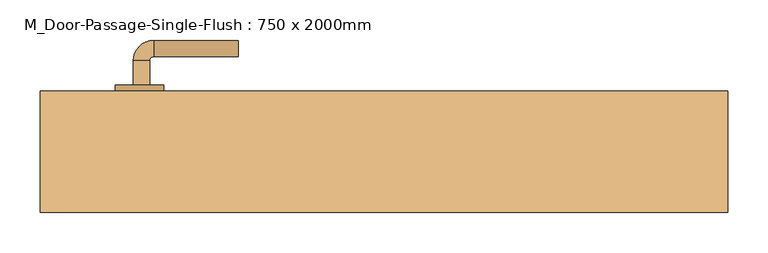
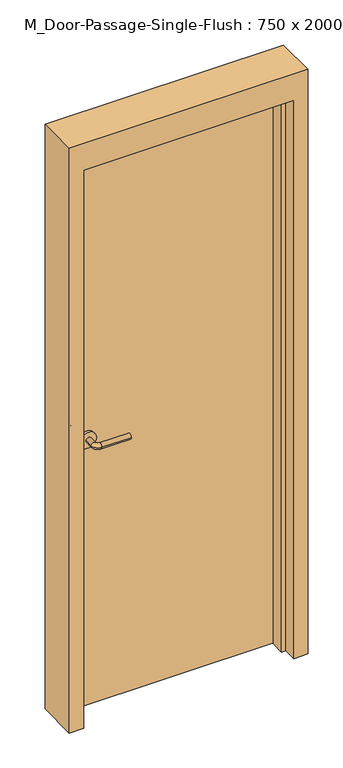
"""IFC4 building model written with IfcOpenShell, lengths in millimetres: door geometry, M_Door-Passage-Single-Flush : 750 x 2000mm."""

from ifc_helpers import new_model, si_unit, point, frame, frame_2d, origin, origin_with_axes, place, context, project, spatial, polyline, circle_curve, ellipse_curve, trimmed, segment, composite_curve, outline, extrude, faceted_brep, source, transform, mapped, element, save
from ifc_brep_helpers import plane_surface, cylinder_surface, revolved_surface, advanced_brep


def m_door_passage_single_flush_750_x_2000mm_58848773(model_context):
    return source(origin(), model_context, "Body", "SolidModel", [
        advanced_brep(
        [(-309.990625, 40.85, 1000.0), (-289.990625, 40.85, 1000.0), (-289.990625, 10.85, 1000.0), (-309.990625, 10.85, 1000.0), (-284.990625, 5.85, 1000.0), (-284.990625, -14.15, 1000.0), (-179.990625, -14.15, 1000.0), (-179.990625, 5.85, 1000.0)],
        [
            (0, 1, circle_curve(frame((-299.990625, 40.85, 1000.0), z_axis=(0.0, 1.0, 0.0), x_axis=(1.0, 0.0, 0.0)), 10.0)),
            (1, 0, circle_curve(frame((-299.990625, 40.85, 1000.0), z_axis=(0.0, 1.0, 0.0), x_axis=(1.0, 0.0, 0.0)), 10.0)),
            (1, 2),
            (2, 3, circle_curve(frame((-299.990625, 10.85, 1000.0), z_axis=(0.0, 1.0, 0.0), x_axis=(1.0, 0.0, 0.0)), 10.0)),
            (3, 0),
            (3, 2, circle_curve(frame((-299.990625, 10.85, 1000.0), z_axis=(0.0, 1.0, 0.0), x_axis=(1.0, 0.0, 0.0)), 10.0)),
            (4, 5, circle_curve(frame((-284.990625, -4.15, 1000.0), z_axis=(-1.0, 0.0, 0.0), x_axis=(0.0, 1.0, 0.0)), 10.0)),
            (5, 3, circle_curve(frame((-284.990625, 10.85, 1000.0), z_axis=(0.0, 0.0, -1.0), x_axis=(-1.0, 0.0, 0.0)), 25.0)),
            (2, 4, circle_curve(frame((-284.990625, 10.85, 1000.0), z_axis=(0.0, 0.0, 1.0), x_axis=(-1.0, 0.0, 0.0)), 5.0)),
            (5, 4, circle_curve(frame((-284.990625, -4.15, 1000.0), z_axis=(-1.0, 0.0, 0.0), x_axis=(0.0, 1.0, 0.0)), 10.0)),
            (6, 7, circle_curve(frame((-179.990625, -4.15, 1000.0), z_axis=(1.0, 0.0, 0.0), x_axis=(0.0, 1.0, 0.0)), 10.0)),
            (7, 6, circle_curve(frame((-179.990625, -4.15, 1000.0), z_axis=(1.0, 0.0, 0.0), x_axis=(0.0, 1.0, 0.0)), 10.0)),
            (4, 7),
            (6, 5),
        ],
        [
            plane_surface(frame((-299.990625, 40.85, 1000.0), z_axis=(0.0, 1.0, 0.0), x_axis=(0.0, 0.0, 1.0))),
            cylinder_surface(frame((-299.990625, 40.85, 1000.0), z_axis=(0.0, 1.0, 0.0), x_axis=(1.0, 0.0, 0.0)), 10.0),
            revolved_surface(trimmed(ellipse_curve(frame((-299.990625, 10.85, 1000.0), z_axis=(0.0, -1.0, 0.0), x_axis=(1.0, 0.0, 0.0)), 10.0, 10.0), [point((-309.990625, 10.85, 1000.0))], [point((-289.990625, 10.85, 1000.0))], True, "CARTESIAN"), (-284.990625, 10.85, 1000.0), (0.0, 0.0, -1.0)),
            revolved_surface(trimmed(ellipse_curve(frame((-299.990625, 10.85, 1000.0), z_axis=(0.0, -1.0, 0.0), x_axis=(1.0, 0.0, 0.0)), 10.0, 10.0), [point((-289.990625, 10.85, 1000.0))], [point((-309.990625, 10.85, 1000.0))], True, "CARTESIAN"), (-284.990625, 10.85, 1000.0), (0.0, 0.0, -1.0)),
            plane_surface(frame((-179.990625, -4.15, 1000.0), z_axis=(1.0, 0.0, 0.0), x_axis=(0.0, 0.0, 1.0))),
            cylinder_surface(frame((-284.990625, -4.15, 1000.0), z_axis=(-1.0, 0.0, 0.0), x_axis=(0.0, 1.0, 0.0)), 10.0),
        ],
        [
            (0, [[1, 2]]),
            (1, [[3, 4, 5, -2]]),
            (1, [[-5, 6, -3, -1]]),
            (2, [[7, 8, -4, 9]]),
            (3, [[10, -9, -6, -8]]),
            (4, [[11, 12]]),
            (5, [[13, -11, 14, -7]]),
            (5, [[-14, -12, -13, -10]]),
        ],
    ),
        extrude(outline(composite_curve([segment(trimmed(circle_curve(frame_2d((1000.0, -302.490625)), 30.0), [point((1000.0, -332.490625))], [point((1000.0, -272.490625))], False, "CARTESIAN"), True, "CONTINUOUS"), segment(trimmed(circle_curve(frame_2d((1000.0, -302.490625)), 30.0), [point((1000.0, -272.490625))], [point((1000.0, -332.490625))], False, "CARTESIAN"), True, "CONTINUOUS")], self_intersect=False)), frame((0.0, 40.85, 0.0), z_axis=(0.0, 1.0, 0.0), x_axis=(0.0, 0.0, 1.0)), (0.0, 0.0, 1.0), 8.0),
        advanced_brep(
        [(-309.990625, 101.85, 1000.0), (-289.990625, 101.85, 1000.0), (-309.990625, 131.85, 1000.0), (-289.990625, 131.85, 1000.0), (-284.990625, 136.85, 1000.0), (-284.990625, 156.85, 1000.0), (-179.990625, 156.85, 1000.0), (-179.990625, 136.85, 1000.0)],
        [
            (0, 1, circle_curve(frame((-299.990625, 101.85, 1000.0), z_axis=(0.0, -1.0, 0.0), x_axis=(1.0, 0.0, 0.0)), 10.0)),
            (1, 0, circle_curve(frame((-299.990625, 101.85, 1000.0), z_axis=(0.0, -1.0, 0.0), x_axis=(1.0, 0.0, 0.0)), 10.0)),
            (0, 2),
            (2, 3, circle_curve(frame((-299.990625, 131.85, 1000.0), z_axis=(0.0, -1.0, 0.0), x_axis=(1.0, 0.0, 0.0)), 10.0)),
            (3, 1),
            (3, 2, circle_curve(frame((-299.990625, 131.85, 1000.0), z_axis=(0.0, -1.0, 0.0), x_axis=(1.0, 0.0, 0.0)), 10.0)),
            (4, 3, circle_curve(frame((-284.990625, 131.85, 1000.0), z_axis=(0.0, 0.0, 1.0), x_axis=(-1.0, 0.0, 0.0)), 5.0)),
            (2, 5, circle_curve(frame((-284.990625, 131.85, 1000.0), z_axis=(0.0, 0.0, -1.0), x_axis=(-1.0, 0.0, 0.0)), 25.0)),
            (5, 4, circle_curve(frame((-284.990625, 146.85, 1000.0), z_axis=(-1.0, 0.0, 0.0), x_axis=(0.0, -1.0, 0.0)), 10.0)),
            (4, 5, circle_curve(frame((-284.990625, 146.85, 1000.0), z_axis=(-1.0, 0.0, 0.0), x_axis=(0.0, -1.0, 0.0)), 10.0)),
            (6, 7, circle_curve(frame((-179.990625, 146.85, 1000.0), z_axis=(1.0, 0.0, 0.0), x_axis=(0.0, -1.0, 0.0)), 10.0)),
            (7, 6, circle_curve(frame((-179.990625, 146.85, 1000.0), z_axis=(1.0, 0.0, 0.0), x_axis=(0.0, -1.0, 0.0)), 10.0)),
            (5, 6),
            (7, 4),
        ],
        [
            plane_surface(frame((-299.990625, 101.85, 1000.0), z_axis=(0.0, -1.0, 0.0), x_axis=(0.0, 0.0, 1.0))),
            cylinder_surface(frame((-299.990625, 101.85, 1000.0), z_axis=(0.0, -1.0, 0.0), x_axis=(1.0, 0.0, 0.0)), 10.0),
            revolved_surface(trimmed(ellipse_curve(frame((-299.990625, 131.85, 1000.0), z_axis=(0.0, -1.0, 0.0), x_axis=(1.0, 0.0, 0.0)), 10.0, 10.0), [point((-309.990625, 131.85, 1000.0))], [point((-289.990625, 131.85, 1000.0))], True, "CARTESIAN"), (-284.990625, 131.85, 1000.0), (0.0, 0.0, -1.0)),
            revolved_surface(trimmed(ellipse_curve(frame((-299.990625, 131.85, 1000.0), z_axis=(0.0, -1.0, 0.0), x_axis=(1.0, 0.0, 0.0)), 10.0, 10.0), [point((-289.990625, 131.85, 1000.0))], [point((-309.990625, 131.85, 1000.0))], True, "CARTESIAN"), (-284.990625, 131.85, 1000.0), (0.0, 0.0, -1.0)),
            plane_surface(frame((-179.990625, 146.85, 1000.0), z_axis=(1.0, 0.0, 0.0), x_axis=(0.0, 0.0, 1.0))),
            cylinder_surface(frame((-284.990625, 146.85, 1000.0), z_axis=(-1.0, 0.0, 0.0), x_axis=(0.0, -1.0, 0.0)), 10.0),
        ],
        [
            (0, [[1, 2]]),
            (1, [[-1, 3, 4, 5]]),
            (1, [[-2, -5, 6, -3]]),
            (2, [[7, -4, 8, 9]]),
            (3, [[-8, -6, -7, 10]]),
            (4, [[11, 12]]),
            (5, [[-9, 13, -12, 14]]),
            (5, [[-10, -14, -11, -13]]),
        ],
    ),
        extrude(outline(composite_curve([segment(trimmed(circle_curve(frame_2d((1000.0, -302.490625)), 30.0), [point((1000.0, -332.490625))], [point((1000.0, -272.490625))], False, "CARTESIAN"), True, "CONTINUOUS"), segment(trimmed(circle_curve(frame_2d((1000.0, -302.490625)), 30.0), [point((1000.0, -272.490625))], [point((1000.0, -332.490625))], False, "CARTESIAN"), True, "CONTINUOUS")], self_intersect=False)), frame((0.0, 93.85, 0.0), z_axis=(0.0, 1.0, 0.0), x_axis=(0.0, 0.0, 1.0)), (0.0, 0.0, 1.0), 8.0),
        extrude(outline(polyline([(375.0, 48.85), (-375.0, 48.85), (-375.0, 93.85), (375.0, 93.85), (375.0, 48.85)])), origin_with_axes(), (0.0, 0.0, 1.0), 2100.0),
        faceted_brep([(375.0, 44.0875, 0.0), (375.0, 93.85, 0.0), (425.0, 93.85, 0.0), (425.0, -56.15, 0.0), (375.0, -56.15, 0.0), (375.0, -6.9375, 0.0), (359.125, -6.9375, 0.0), (359.125, 44.0875, 0.0), (375.0, 44.0875, 2100.0), (375.0, 93.85, 2100.0), (-375.0, 93.85, 2100.0), (-375.0, 93.85, 0.0), (-425.0, 93.85, 0.0), (-425.0, 93.85, 2200.0), (425.0, 93.85, 2200.0), (425.0, -56.15, 2200.0), (-425.0, -56.15, 2200.0), (-425.0, -56.15, 0.0), (-375.0, -56.15, 0.0), (-375.0, -56.15, 2100.0), (375.0, -56.15, 2100.0), (375.0, -6.9375, 2100.0), (-375.0, -6.9375, 2100.0), (-375.0, -6.9375, 0.0), (-359.125, -6.9375, 0.0), (-359.125, -6.9375, 2084.125), (359.125, -6.9375, 2084.125), (359.125, 44.0875, 2084.125), (-359.125, 44.0875, 2084.125), (-359.125, 44.0875, 0.0), (-375.0, 44.0875, 0.0), (-375.0, 44.0875, 2100.0)], [[[0, 1, 2, 3, 4, 5, 6, 7]], [[1, 0, 8, 9]], [[2, 1, 9, 10, 11, 12, 13, 14]], [[3, 2, 14, 15]], [[4, 3, 15, 16, 17, 18, 19, 20]], [[5, 4, 20, 21]], [[6, 5, 21, 22, 23, 24, 25, 26]], [[7, 6, 26, 27]], [[0, 7, 27, 28, 29, 30, 31, 8]], [[9, 8, 31, 10]], [[20, 19, 22, 21]], [[26, 25, 28, 27]], [[12, 11, 30, 29, 24, 23, 18, 17]], [[11, 10, 31, 30]], [[13, 12, 17, 16]], [[19, 18, 23, 22]], [[25, 24, 29, 28]], [[15, 14, 13, 16]]]),
    ])


if __name__ == "__main__":
    model = new_model("IFC4")
    model_context = context("Model", 3, world=origin())
    ifc_project = project(units=[si_unit("LENGTHUNIT", "METRE", prefix="MILLI")], contexts=[model_context])
    site = spatial("IfcSite", under=ifc_project)
    building = spatial("IfcBuilding", under=site)
    placement = place(None, origin())
    m_door_passage_single_flush_750_x_2000mm_shape = m_door_passage_single_flush_750_x_2000mm_58848773(model_context)
    element("IfcDoor", 1, ObjectType="M_Door-Passage-Single-Flush : 750 x 2000mm", at=placement, inside=building, context=model_context, shape_type="MappedRepresentation", body=[
        mapped(m_door_passage_single_flush_750_x_2000mm_shape, transform((0.0, 0.0, 0.0), x_axis=(1.0, 0.0, 0.0), y_axis=(0.0, 1.0, 0.0), z_axis=(0.0, 0.0, 1.0))),
    ])
    save(model, "model.ifc")

# Revit data of these elements
# Type "M_Door-Passage-Single-Flush : 750 x 2000mm"
#   Type Mark = "35"
#   Assembly Code = "B2030200"
#   Analytic Construction = "Wooden"
#   Thickness = 45 mm
#   Thermal Resistance (R) = 0.455703 (m²·K)/W
#   Swing Angle [instance default] = 90.00°
#   Strike Height = 1000 mm
#   Rough Width [instance default] = 850 mm
#   Rough Height [instance default] = 2200 mm
#   MF Opening Height [instance default] = 100 mm
#   MF Opening Width [instance default] = 100 mm
#   Inset Calculate [instance default] = 105 mm
#   Masonry Inset [instance default] = 25 mm
#   Height = 2100 mm
#   Width = 750 mm
#   Heat Transfer Coefficient (U) = 2.19465 W/(m²·K)
#   Masonry Frame Depth = 150 mm
#   Masonry Frame [instance default] = yes
#   Function = 1
#   Dry Wall Frame [instance default] = no
#   Panel Material = Wood - Birch
#   Frame Material = Metal - Paint Finish - Grey
#   Door Handle Material = Aluminum
#   Visual Light Transmittance = 0
#   Solar Heat Gain Coefficient = 0
#   Wall Closure = (empty or 0)
# Element 1 (IfcDoor, "M_Door-Passage-Single-Flush : 750 x 2000mm")
#   Materials on its faces: "Aluminum", "Metal - Paint Finish - Grey", "Wood - Birch"
# Materials
#   "Wood - Birch": class "Wood", colour RGB 173 132 96, transparency 0, Cost = 0
#   "Metal - Paint Finish - Grey": class "Paint", colour RGB 178 178 178, transparency 0, Cost = 0
#   "Aluminum": class "Metal", colour RGB 244 245 246, transparency 0, Description = "Aluminum 6061", Cost = 0
